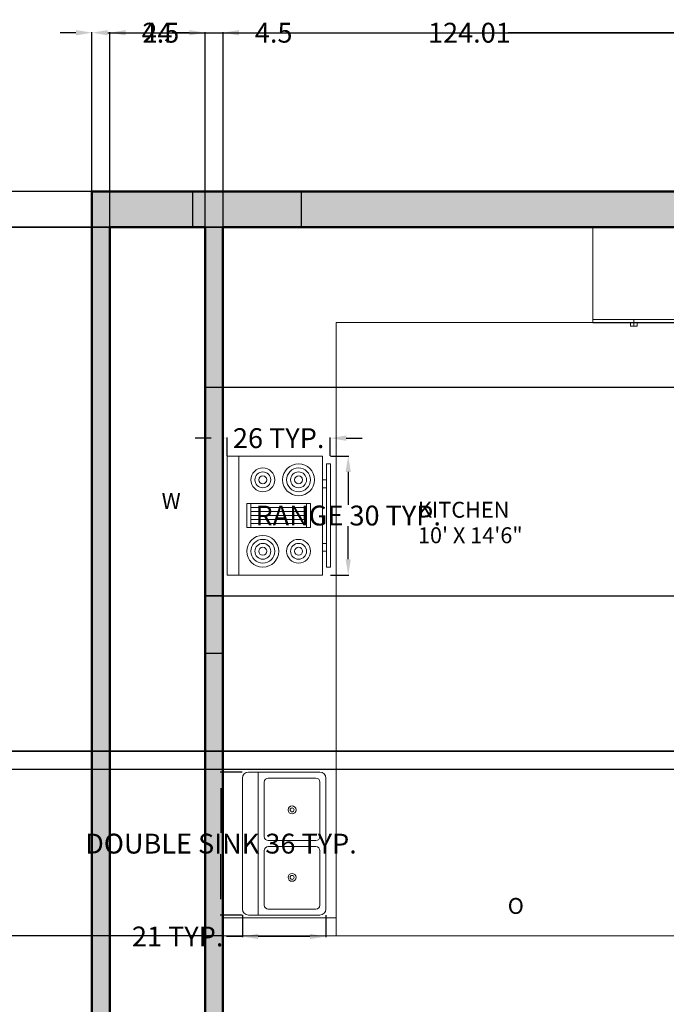
# Model space of a CAD drawing. Units: inches. Extents: x -12 to 887, y 330 to 874.
# Tile 7 of 9: x 442 to 605, y 626 to 874. Entities that reach past the tile are written whole.
import ezdxf

# ---------------------------------------------------------------- set-up
doc = ezdxf.new("R2010")
doc.units = ezdxf.units.IN
doc.header["$MEASUREMENT"] = 0
for name, color, linetype, lineweight in [('A-ANNO-DIMS', 2, 'Continuous', 18), ('A-ANNO-TEXT', 3, 'Continuous', 18), ('A-AREA-IDEN', 7, 'Continuous', 18), ('A-EQPM', 8, 'Continuous', 18), ('A-FLOR-FIXT', 8, 'Continuous', 18), ('A-GLAZ', 4, 'Continuous', 25), ('A-WALL', 7, 'Continuous', 50), ('A-WALL-PATT', 5, 'Continuous', 13)]:
    doc.layers.add(name, color=color, linetype=linetype, lineweight=lineweight)
doc.styles.get("Standard").update_dxf_attribs({"font": 'arial.ttf'})
doc.dimstyles.get("Standard").update_dxf_attribs({"dimtxt": 5, "dimasz": 4, "dimexe": 0.18, "dimexo": 0.0625, "dimgap": 0.09, "dimtad": 0, "dimtih": 1, "dimtoh": 1, "dimdec": 1, "dimzin": 0, "dimdsep": 46, "dimlunit": 4, "dimtxsty": 'Standard', "dimcen": 0.09, "dimadec": 0, "dimazin": 0, "dimtfac": 1, "dimtdec": 1, "dimtofl": 0, "dimtmove": 0, "dimatfit": 3, "dimfxl": 1, "dimtolj": 1, "dimtzin": 0, "dimarcsym": 0})

# ---------------------------------------------------------------- blocks, each defined once
blk = doc.blocks.new('Sink-double - 36 in top')
for p, q in [((-18, -4), (18, -4)), ((-0.75, -18.5), (-0.75, -6.5)), ((0.75, -6.5), (0.75, -18.5))]:
    blk.add_line(p, q)
for points in [[(-16.5, 0), (16.5, 0)], [(-18, -19.5), (-18, -1.5)], [(18, -1.5), (18, -19.5)], [(-16.5, -18.5), (-16.5, -6.5)], [(-15.5, -5.5), (-1.75, -5.5)], [(1.75, -5.5), (15.5, -5.5)], [(16.5, -6.5), (16.5, -18.5)], [(-1.75, -19.5), (-15.5, -19.5)], [(15.5, -19.5), (1.75, -19.5)], [(16.5, -21), (-16.5, -21)]]:
    blk.add_lwpolyline(points)
for centre, radius in [((-8.5, -12.5), 1), ((-8.5, -12.5), 0.5), ((8.5, -12.5), 1), ((8.5, -12.5), 0.5)]:
    blk.add_circle(centre, radius)
for centre, radius, start, end in [((-16.5, -1.5), 1.5, 90, 180), ((16.5, -1.5), 1.5, 0, 90), ((-15.5, -6.5), 1, 90, 180), ((-1.75, -6.5), 1, 0, 90), ((1.75, -6.5), 1, 90, 180), ((15.5, -6.5), 1, 0, 90), ((-16.5, -19.5), 1.5, 180, 270), ((-15.5, -18.5), 1, 180, 270), ((-1.75, -18.5), 1, 270, 0), ((1.75, -18.5), 1, 180, 270), ((15.5, -18.5), 1, 270, 0), ((16.5, -19.5), 1.5, 270, 0)]:
    blk.add_arc(centre, radius, start, end)
blk = doc.blocks.new('Range-Oven - 30 in top')
for p, q in [((0, -3), (30, -3)), ((12, -6), (18, -6)), ((13, -20), (13, -6)), ((14, -6), (14, -20)), ((15, -20), (15, -6)), ((16, -6), (16, -20)), ((17, -20), (17, -6)), ((18, -20), (12, -20)), ((6, -24), (6, -25)), ((8, -25), (8, -24)), ((22, -25), (22, -24)), ((24, -24), (24, -25))]:
    blk.add_line(p, q)
for points in [[(0, -24), (0, 0), (30, 0), (30, -24)], [(12, -21), (12, -5), (18, -5), (18, -21)], [(2, -26), (2, -25), (28, -25), (28, -26)]]:
    blk.add_lwpolyline(points, close=True)
for centre, radius in [((6, -9), 4), ((6, -9), 3), ((6, -9), 2), ((24, -9), 3), ((24, -9), 2), ((6, -9), 1), ((24, -9), 1), ((24, -18), 4), ((6, -18), 3), ((6, -18), 2), ((6, -18), 1), ((24, -18), 3), ((24, -18), 2), ((24, -18), 1)]:
    blk.add_circle(centre, radius)
blk = doc.blocks.new('Refrigerator-2 door - 36 in top')
for p, q in [((0, -26.999999), (36, -26.999999)), ((11, -27.999999), (11, -28.999999)), ((12, -26.999999), (12, -28.999999)), ((13, -28.999999), (13, -27.999999)), ((11, -28.999999), (13, -28.999999))]:
    blk.add_line(p, q)
blk.add_lwpolyline([(0, -27.999999), (0, 0), (36, 0), (36, -27.999999)], close=True)
blk = doc.blocks.new('*D24')
at = {"layer": 'A-ANNO-DIMS', "color": 0, "lineweight": -2, "transparency": 16777216}
for p, q in [((497.9, 684.39), (492.38, 684.39)), ((492.56, 680.39), (492.56, 669.07)), ((492.56, 652.39), (492.56, 663.71)), ((497.9, 648.39), (492.38, 648.39))]:
    blk.add_line(p, q, dxfattribs=at)
at = {"layer": 'A-ANNO-DIMS', "color": 0, "transparency": 16777216}
for points in [[(491.89, 680.39), (493.23, 680.39), (492.56, 684.39)], [(491.89, 652.39), (493.23, 652.39), (492.56, 648.39)]]:
    blk.add_solid(points, dxfattribs=at)
at = {"layer": 'Defpoints', "color": 0, "transparency": 16777216}
for p in [(492.56, 684.39), (497.96, 684.39), (497.96, 648.39)]:
    blk.add_point(p, dxfattribs=at)
at = {"layer": 'A-ANNO-DIMS', "color": 0, "transparency": 16777216, "insert": (492.56, 666.39), "char_height": 5, "attachment_point": 5}
blk.add_mtext('\\A1;DOUBLE SINK 36 TYP.', dxfattribs=at)
blk = doc.blocks.new('*D25')
at = {"layer": 'A-ANNO-DIMS', "color": 0, "lineweight": -2, "transparency": 16777216}
for p, q in [((497.96, 648.33), (497.96, 642.81)), ((518.96, 648.33), (518.96, 642.81)), ((497.96, 642.99), (493.96, 642.99)), ((514.96, 642.99), (501.96, 642.99))]:
    blk.add_line(p, q, dxfattribs=at)
at = {"layer": 'A-ANNO-DIMS', "color": 0, "transparency": 16777216}
for points in [[(501.96, 643.66), (501.96, 642.33), (497.96, 642.99)], [(514.96, 643.66), (514.96, 642.33), (518.96, 642.99)]]:
    blk.add_solid(points, dxfattribs=at)
at = {"layer": 'Defpoints', "color": 0, "transparency": 16777216}
for p in [(497.96, 648.39), (518.96, 648.39), (497.96, 642.99)]:
    blk.add_point(p, dxfattribs=at)
at = {"layer": 'A-ANNO-DIMS', "color": 0, "transparency": 16777216, "insert": (481.66, 642.99), "char_height": 5, "attachment_point": 5}
blk.add_mtext('\\A1;21 TYP.', dxfattribs=at)
blk = doc.blocks.new('*D26')
at = {"layer": 'A-ANNO-DIMS', "color": 0, "lineweight": -2, "transparency": 16777216}
for p, q in [((520.15, 764.03), (524.76, 764.03)), ((524.58, 760.03), (524.58, 751.71)), ((524.58, 738.03), (524.58, 746.35)), ((520.15, 734.03), (524.76, 734.03))]:
    blk.add_line(p, q, dxfattribs=at)
at = {"layer": 'A-ANNO-DIMS', "color": 0, "transparency": 16777216}
for points in [[(523.92, 760.03), (525.25, 760.03), (524.58, 764.03)], [(523.92, 738.03), (525.25, 738.03), (524.58, 734.03)]]:
    blk.add_solid(points, dxfattribs=at)
at = {"layer": 'Defpoints', "color": 0, "transparency": 16777216}
for p in [(520.08, 764.03), (524.58, 764.03), (520.08, 734.03)]:
    blk.add_point(p, dxfattribs=at)
at = {"layer": 'A-ANNO-DIMS', "color": 0, "transparency": 16777216, "insert": (524.58, 749.03), "char_height": 5, "attachment_point": 5}
blk.add_mtext('\\A1;RANGE 30 TYP.', dxfattribs=at)
blk = doc.blocks.new('*D27')
at = {"layer": 'A-ANNO-DIMS', "color": 0, "lineweight": -2, "transparency": 16777216}
for p, q in [((490.08, 768.53), (486.08, 768.53)), ((494.08, 764.09), (494.08, 768.71)), ((520.08, 764.09), (520.08, 768.71)), ((524.08, 768.53), (528.08, 768.53))]:
    blk.add_line(p, q, dxfattribs=at)
at = {"layer": 'A-ANNO-DIMS', "color": 0, "transparency": 16777216}
for points in [[(490.08, 769.2), (490.08, 767.86), (494.08, 768.53)], [(524.08, 769.2), (524.08, 767.86), (520.08, 768.53)]]:
    blk.add_solid(points, dxfattribs=at)
at = {"layer": 'Defpoints', "color": 0, "transparency": 16777216}
for p in [(494.08, 768.53), (494.08, 764.03), (520.08, 764.03)]:
    blk.add_point(p, dxfattribs=at)
at = {"layer": 'A-ANNO-DIMS', "color": 0, "transparency": 16777216, "insert": (507.08, 768.53), "char_height": 5, "attachment_point": 5}
blk.add_mtext('\\A1;26 TYP.', dxfattribs=at)
blk = doc.blocks.new('*D64')
at = {"layer": 'A-ANNO-DIMS', "color": 0, "lineweight": -2, "transparency": 16777216}
for p, q in [((383.99, 685.16), (873.75, 685.16)), ((873.57, 681.16), (873.57, 628.55)), ((873.57, 570.66), (873.57, 623.27)), ((383.99, 566.66), (873.75, 566.66))]:
    blk.add_line(p, q, dxfattribs=at)
at = {"layer": 'A-ANNO-DIMS', "color": 0, "transparency": 16777216}
for points in [[(872.9, 681.16), (874.24, 681.16), (873.57, 685.16)], [(872.9, 570.66), (874.24, 570.66), (873.57, 566.66)]]:
    blk.add_solid(points, dxfattribs=at)
at = {"layer": 'Defpoints', "color": 0, "transparency": 16777216}
for p in [(383.93, 685.16), (873.57, 685.16), (383.93, 566.66)]:
    blk.add_point(p, dxfattribs=at)
at = {"layer": 'A-ANNO-DIMS', "color": 0, "transparency": 16777216, "insert": (873.57, 625.91), "char_height": 5, "attachment_point": 5}
blk.add_mtext('\\A1;118.5', dxfattribs=at)
blk = doc.blocks.new('*D65')
at = {"layer": 'A-ANNO-DIMS', "color": 0, "lineweight": -2, "transparency": 16777216}
for p, q in [((873.57, 693.66), (873.57, 697.66)), ((873.57, 697.66), (877.57, 697.66)), ((383.99, 689.66), (873.75, 689.66)), ((383.99, 685.16), (873.75, 685.16)), ((873.57, 681.16), (873.57, 677.16))]:
    blk.add_line(p, q, dxfattribs=at)
at = {"layer": 'A-ANNO-DIMS', "color": 0, "transparency": 16777216}
for points in [[(872.9, 693.66), (874.24, 693.66), (873.57, 689.66)], [(872.9, 681.16), (874.24, 681.16), (873.57, 685.16)]]:
    blk.add_solid(points, dxfattribs=at)
at = {"layer": 'Defpoints', "color": 0, "transparency": 16777216}
for p in [(383.93, 689.66), (873.57, 689.66), (383.93, 685.16)]:
    blk.add_point(p, dxfattribs=at)
at = {"layer": 'A-ANNO-DIMS', "color": 0, "transparency": 16777216, "insert": (882.33, 697.66), "char_height": 5, "attachment_point": 5}
blk.add_mtext('\\A1;4.5', dxfattribs=at)
blk = doc.blocks.new('*D66')
at = {"layer": 'A-ANNO-DIMS', "color": 0, "lineweight": -2, "transparency": 16777216}
for p, q in [((383.99, 821.66), (873.75, 821.66)), ((873.57, 817.66), (873.57, 758.31)), ((873.57, 693.66), (873.57, 753.02)), ((383.99, 689.66), (873.75, 689.66))]:
    blk.add_line(p, q, dxfattribs=at)
at = {"layer": 'A-ANNO-DIMS', "color": 0, "transparency": 16777216}
for points in [[(872.9, 817.66), (874.24, 817.66), (873.57, 821.66)], [(872.9, 693.66), (874.24, 693.66), (873.57, 689.66)]]:
    blk.add_solid(points, dxfattribs=at)
at = {"layer": 'Defpoints', "color": 0, "transparency": 16777216}
for p in [(383.93, 821.66), (873.57, 821.66), (383.93, 689.66)]:
    blk.add_point(p, dxfattribs=at)
at = {"layer": 'A-ANNO-DIMS', "color": 0, "transparency": 16777216, "insert": (873.57, 755.66), "char_height": 5, "attachment_point": 5}
blk.add_mtext('\\A1;132', dxfattribs=at)
blk = doc.blocks.new('*D83')
at = {"layer": 'A-ANNO-DIMS', "color": 0, "lineweight": -2, "transparency": 16777216}
for p, q in [((460.07, 830.72), (460.07, 870.84)), ((464.07, 870.66), (638.28, 870.66)), ((829.57, 870.66), (655.36, 870.66)), ((833.57, 830.72), (833.57, 870.84))]:
    blk.add_line(p, q, dxfattribs=at)
at = {"layer": 'A-ANNO-DIMS', "color": 0, "transparency": 16777216}
for points in [[(464.07, 871.33), (464.07, 869.99), (460.07, 870.66)], [(829.57, 871.33), (829.57, 869.99), (833.57, 870.66)]]:
    blk.add_solid(points, dxfattribs=at)
at = {"layer": 'Defpoints', "color": 0, "transparency": 16777216}
for p in [(833.57, 870.66), (460.07, 830.66), (833.57, 830.66)]:
    blk.add_point(p, dxfattribs=at)
at = {"layer": 'A-ANNO-DIMS', "color": 0, "transparency": 16777216, "insert": (646.82, 870.66), "char_height": 5, "attachment_point": 5}
blk.add_mtext('\\A1;373.5', dxfattribs=at)
blk = doc.blocks.new('*D84')
at = {"layer": 'A-ANNO-DIMS', "color": 0, "lineweight": -2, "transparency": 16777216}
for p, q in [((456.07, 870.66), (452.07, 870.66)), ((460.07, 830.72), (460.07, 870.84)), ((464.57, 821.72), (464.57, 870.84)), ((468.57, 870.66), (472.57, 870.66))]:
    blk.add_line(p, q, dxfattribs=at)
at = {"layer": 'A-ANNO-DIMS', "color": 0, "transparency": 16777216}
for points in [[(456.07, 871.33), (456.07, 869.99), (460.07, 870.66)], [(468.57, 871.33), (468.57, 869.99), (464.57, 870.66)]]:
    blk.add_solid(points, dxfattribs=at)
at = {"layer": 'Defpoints', "color": 0, "transparency": 16777216}
for p in [(464.57, 870.66), (460.07, 830.66), (464.57, 821.66)]:
    blk.add_point(p, dxfattribs=at)
at = {"layer": 'A-ANNO-DIMS', "color": 0, "transparency": 16777216, "insert": (477.33, 870.66), "char_height": 5, "attachment_point": 5}
blk.add_mtext('\\A1;4.5', dxfattribs=at)
blk = doc.blocks.new('*D85')
at = {"layer": 'A-ANNO-DIMS', "color": 0, "lineweight": -2, "transparency": 16777216}
for p, q in [((464.57, 821.72), (464.57, 870.84)), ((468.57, 870.66), (472.86, 870.66)), ((484.57, 870.66), (480.27, 870.66)), ((488.57, 821.72), (488.57, 870.84))]:
    blk.add_line(p, q, dxfattribs=at)
at = {"layer": 'A-ANNO-DIMS', "color": 0, "transparency": 16777216}
for points in [[(468.57, 871.33), (468.57, 869.99), (464.57, 870.66)], [(484.57, 871.33), (484.57, 869.99), (488.57, 870.66)]]:
    blk.add_solid(points, dxfattribs=at)
at = {"layer": 'Defpoints', "color": 0, "transparency": 16777216}
for p in [(488.57, 870.66), (464.57, 821.66), (488.57, 821.66)]:
    blk.add_point(p, dxfattribs=at)
at = {"layer": 'A-ANNO-DIMS', "color": 0, "transparency": 16777216, "insert": (476.57, 870.66), "char_height": 5, "attachment_point": 5}
blk.add_mtext('\\A1;24', dxfattribs=at)
blk = doc.blocks.new('*D86')
at = {"layer": 'A-ANNO-DIMS', "color": 0, "lineweight": -2, "transparency": 16777216}
for p, q in [((484.57, 870.66), (480.57, 870.66)), ((488.57, 821.72), (488.57, 870.84)), ((493.07, 821.72), (493.07, 870.84)), ((497.07, 870.66), (501.07, 870.66))]:
    blk.add_line(p, q, dxfattribs=at)
at = {"layer": 'A-ANNO-DIMS', "color": 0, "transparency": 16777216}
for points in [[(484.57, 871.33), (484.57, 869.99), (488.57, 870.66)], [(497.07, 871.33), (497.07, 869.99), (493.07, 870.66)]]:
    blk.add_solid(points, dxfattribs=at)
at = {"layer": 'Defpoints', "color": 0, "transparency": 16777216}
for p in [(493.07, 870.66), (488.57, 821.66), (493.07, 821.66)]:
    blk.add_point(p, dxfattribs=at)
at = {"layer": 'A-ANNO-DIMS', "color": 0, "transparency": 16777216, "insert": (505.83, 870.66), "char_height": 5, "attachment_point": 5}
blk.add_mtext('\\A1;4.5', dxfattribs=at)
blk = doc.blocks.new('*D87')
at = {"layer": 'A-ANNO-DIMS', "color": 0, "lineweight": -2, "transparency": 16777216}
for p, q in [((493.07, 821.72), (493.07, 870.84)), ((497.07, 870.66), (545.32, 870.66)), ((613.08, 870.66), (564.83, 870.66)), ((617.08, 821.7), (617.08, 870.84))]:
    blk.add_line(p, q, dxfattribs=at)
at = {"layer": 'A-ANNO-DIMS', "color": 0, "transparency": 16777216}
for points in [[(497.07, 871.33), (497.07, 869.99), (493.07, 870.66)], [(613.08, 871.33), (613.08, 869.99), (617.08, 870.66)]]:
    blk.add_solid(points, dxfattribs=at)
at = {"layer": 'Defpoints', "color": 0, "transparency": 16777216}
for p in [(617.08, 870.66), (493.07, 821.66), (617.08, 821.64)]:
    blk.add_point(p, dxfattribs=at)
at = {"layer": 'A-ANNO-DIMS', "color": 0, "transparency": 16777216, "insert": (555.08, 870.66), "char_height": 5, "attachment_point": 5}
blk.add_mtext('\\A1;124.01', dxfattribs=at)
blk = doc.blocks.new('*D98')
at = {"layer": 'A-ANNO-DIMS', "color": 0, "lineweight": -2, "transparency": 16777216}
for p, q in [((460.13, 830.66), (873.75, 830.66)), ((873.57, 826.66), (873.57, 604.54)), ((873.57, 377.16), (873.57, 599.28)), ((460.13, 373.16), (873.75, 373.16))]:
    blk.add_line(p, q, dxfattribs=at)
at = {"layer": 'A-ANNO-DIMS', "color": 0, "transparency": 16777216}
for points in [[(872.9, 826.66), (874.24, 826.66), (873.57, 830.66)], [(872.9, 377.16), (874.24, 377.16), (873.57, 373.16)]]:
    blk.add_solid(points, dxfattribs=at)
at = {"layer": 'Defpoints', "color": 0, "transparency": 16777216}
for p in [(460.07, 830.66), (873.57, 830.66), (460.07, 373.16)]:
    blk.add_point(p, dxfattribs=at)
at = {"layer": 'A-ANNO-DIMS', "color": 0, "transparency": 16777216, "insert": (873.57, 601.91), "char_height": 5, "attachment_point": 5}
blk.add_mtext('\\A1;457.5', dxfattribs=at)
blk = doc.blocks.new('*D101')
at = {"layer": 'A-ANNO-DIMS', "color": 0, "lineweight": -2, "transparency": 16777216}
for p, q in [((493.01, 643.16), (1.75, 643.16)), ((1.93, 639.16), (1.93, 551.3)), ((1.93, 458.16), (1.93, 546.02)), ((493.01, 454.16), (1.75, 454.16))]:
    blk.add_line(p, q, dxfattribs=at)
at = {"layer": 'A-ANNO-DIMS', "color": 0, "transparency": 16777216}
for points in [[(1.26, 639.16), (2.59, 639.16), (1.93, 643.16)], [(1.26, 458.16), (2.59, 458.16), (1.93, 454.16)]]:
    blk.add_solid(points, dxfattribs=at)
at = {"layer": 'Defpoints', "color": 0, "transparency": 16777216}
for p in [(1.93, 643.16), (493.07, 643.16), (493.07, 454.16)]:
    blk.add_point(p, dxfattribs=at)
at = {"layer": 'A-ANNO-DIMS', "color": 0, "transparency": 16777216, "insert": (1.93, 548.66), "char_height": 5, "attachment_point": 5}
blk.add_mtext('\\A1;189', dxfattribs=at)
blk = doc.blocks.new('*D102')
at = {"layer": 'A-ANNO-DIMS', "color": 0, "lineweight": -2, "transparency": 16777216}
for p, q in [((493.01, 821.66), (1.75, 821.66)), ((1.93, 817.66), (1.93, 735.05)), ((1.93, 647.16), (1.93, 729.77)), ((493.01, 643.16), (1.75, 643.16))]:
    blk.add_line(p, q, dxfattribs=at)
at = {"layer": 'A-ANNO-DIMS', "color": 0, "transparency": 16777216}
for points in [[(1.26, 817.66), (2.59, 817.66), (1.93, 821.66)], [(1.26, 647.16), (2.59, 647.16), (1.93, 643.16)]]:
    blk.add_solid(points, dxfattribs=at)
at = {"layer": 'Defpoints', "color": 0, "transparency": 16777216}
for p in [(1.93, 821.66), (493.07, 821.66), (493.07, 643.16)]:
    blk.add_point(p, dxfattribs=at)
at = {"layer": 'A-ANNO-DIMS', "color": 0, "transparency": 16777216, "insert": (1.93, 732.41), "char_height": 5, "attachment_point": 5}
blk.add_mtext('\\A1;178.5', dxfattribs=at)
blk = doc.blocks.new('*D103')
at = {"layer": 'A-ANNO-DIMS', "color": 0, "lineweight": -2, "transparency": 16777216}
for p, q in [((1.93, 830.66), (1.93, 834.66)), ((1.93, 834.66), (5.93, 834.66)), ((460.01, 830.66), (1.75, 830.66)), ((1.93, 825.66), (1.93, 826.66)), ((493.01, 821.66), (1.75, 821.66))]:
    blk.add_line(p, q, dxfattribs=at)
at = {"layer": 'A-ANNO-DIMS', "color": 0, "transparency": 16777216}
for points in [[(1.26, 826.66), (2.59, 826.66), (1.93, 830.66)], [(1.26, 825.66), (2.59, 825.66), (1.93, 821.66)]]:
    blk.add_solid(points, dxfattribs=at)
at = {"layer": 'Defpoints', "color": 0, "transparency": 16777216}
for p in [(1.93, 830.66), (460.07, 830.66), (493.07, 821.66)]:
    blk.add_point(p, dxfattribs=at)
at = {"layer": 'A-ANNO-DIMS', "color": 0, "transparency": 16777216, "insert": (7.66, 834.66), "char_height": 5, "attachment_point": 5}
blk.add_mtext('\\A1;9', dxfattribs=at)
blk = doc.blocks.new('*D112')
at = {"layer": 'A-ANNO-DIMS', "color": 0, "lineweight": -2, "transparency": 16777216}
for p, q in [((676.01, 821.66), (1.75, 821.66)), ((1.93, 817.66), (1.93, 758.31)), ((1.93, 693.66), (1.93, 753.02)), ((676.01, 689.66), (1.75, 689.66))]:
    blk.add_line(p, q, dxfattribs=at)
at = {"layer": 'A-ANNO-DIMS', "color": 0, "transparency": 16777216}
for points in [[(1.26, 817.66), (2.59, 817.66), (1.93, 821.66)], [(1.26, 693.66), (2.59, 693.66), (1.93, 689.66)]]:
    blk.add_solid(points, dxfattribs=at)
at = {"layer": 'Defpoints', "color": 0, "transparency": 16777216}
for p in [(1.93, 821.66), (676.07, 821.66), (676.07, 689.66)]:
    blk.add_point(p, dxfattribs=at)
at = {"layer": 'A-ANNO-DIMS', "color": 0, "transparency": 16777216, "insert": (1.93, 755.66), "char_height": 5, "attachment_point": 5}
blk.add_mtext('\\A1;132', dxfattribs=at)
blk = doc.blocks.new('*D128')
at = {"layer": 'A-ANNO-DIMS', "color": 0, "lineweight": -2, "transparency": 16777216}
for p, q in [((488.63, 781.36), (873.75, 781.36)), ((873.57, 777.36), (873.57, 757.74)), ((873.57, 732.83), (873.57, 752.45)), ((488.63, 728.83), (873.75, 728.83))]:
    blk.add_line(p, q, dxfattribs=at)
at = {"layer": 'A-ANNO-DIMS', "color": 0, "transparency": 16777216}
for points in [[(872.9, 777.36), (874.24, 777.36), (873.57, 781.36)], [(872.9, 732.83), (874.24, 732.83), (873.57, 728.83)]]:
    blk.add_solid(points, dxfattribs=at)
at = {"layer": 'Defpoints', "color": 0, "transparency": 16777216}
for p in [(488.57, 781.36), (488.57, 728.83), (873.57, 728.83)]:
    blk.add_point(p, dxfattribs=at)
at = {"layer": 'A-ANNO-DIMS', "color": 0, "transparency": 16777216, "insert": (873.57, 755.1), "char_height": 5, "attachment_point": 5}
blk.add_mtext('\\A1;52.54', dxfattribs=at)

msp = doc.modelspace()

# ---------------------------------------------------------------- hatches: boundary and pattern name
at = {"layer": 'A-WALL-PATT'}
h = msp.add_hatch(color=256, dxfattribs=at)
h.dxf.hatch_style = 1
h.paths.add_polyline_path([(94.575, 830.6611), (67.3199, 830.6611), (67.3199, 821.6611), (70.4263, 821.6611), (79.4263, 821.6611), (94.575, 821.6611)])
h.paths.add_polyline_path([(288.8031, 830.6611), (257.9263, 830.6611), (253.4263, 830.6611), (253.4263, 821.6611), (288.8031, 821.6611)])
h.paths.add_polyline_path([(74.9263, 696.9265), (70.4263, 696.9265), (70.4263, 678.4656), (74.9263, 678.4656)])
h.paths.add_polyline_path([(74.9263, 584.8756), (70.4263, 584.8756), (70.4263, 562.1611), (74.9263, 562.1611)])
h.paths.add_polyline_path([(135.5357, 566.6611), (122.6994, 566.6611), (122.6994, 562.1611), (135.5357, 562.1611)])
h.paths.add_polyline_path([(257.9263, 579.1607), (253.4263, 579.1607), (253.4263, 562.1611), (257.9263, 562.1611)])
h.paths.add_polyline_path([(272.0195, 454.1611), (254.2006, 454.1611), (254.2006, 450.1611), (272.0195, 450.1611)])
h.paths.add_polyline_path([(392.9263, 454.1611), (374.959, 454.1611), (374.959, 450.1611), (383.9263, 450.1611), (392.9263, 450.1611)])
h.paths.add_polyline_path([(493.0683, 466.4171), (488.5683, 466.4171), (488.5683, 450.1611), (493.0683, 450.1611)])
h.paths.add_polyline_path([(568.6302, 454.1611), (555.938, 454.1611), (555.938, 450.1611), (568.6302, 450.1611)])
h.paths.add_polyline_path([(493.0683, 594.9471), (488.5683, 594.9471), (488.5683, 569.5862), (493.0683, 569.5862)])
h.paths.add_polyline_path([(690.1615, 454.1611), (672.3426, 454.1611), (672.3426, 450.1611), (690.1615, 450.1611)])
h.paths.add_polyline_path([(811.0683, 454.1611), (793.101, 454.1611), (793.101, 450.1611), (802.0683, 450.1611), (811.0683, 450.1611)])
h.paths.add_polyline_path([(811.0683, 578.3606), (802.0683, 578.3606), (802.0683, 566.6611), (802.0683, 553.5254), (811.0683, 553.5254)])
h.paths.add_polyline_path([(811.0683, 701.6611), (802.0683, 701.6611), (802.0683, 689.9616), (802.0683, 676.8259), (811.0683, 676.8259)])
h.paths.add_polyline_path([(811.0683, 830.6611), (782.165, 830.6611), (782.165, 821.6611), (802.0683, 821.6611), (811.0683, 821.6611)])
h.paths.add_polyline_path([(706.9451, 830.6611), (671.5683, 830.6611), (671.5683, 821.6611), (706.9451, 821.6611)])
h.paths.add_polyline_path([(512.717, 830.6611), (485.4619, 830.6611), (485.4619, 821.6611), (488.5683, 821.6611), (512.717, 821.6611)])
h.paths.add_polyline_path([(392.9263, 697.8668), (383.9263, 697.8668), (383.9263, 689.6611), (383.9263, 676.5034), (392.9263, 676.5034)])
h.paths.add_polyline_path([(392.9263, 830.6611), (364.023, 830.6611), (364.023, 821.7357), (392.9263, 821.7357)])
h.paths.add_polyline_path([(392.9263, 619.0434), (383.9263, 619.0434), (383.9263, 588.7499), (392.9263, 588.7499)])
h.paths.add_polyline_path([(392.9263, 578.3606), (383.9263, 578.3606), (383.9263, 566.6611), (383.9263, 553.5254), (392.9263, 553.5254)])
h.paths.add_polyline_path([(257.9263, 699.8547), (253.4263, 699.8547), (253.4263, 697.1611), (253.4263, 677.338), (257.9263, 677.338)])
h.paths.add_polyline_path([(493.0683, 714.3785), (488.5683, 714.3785), (488.5683, 689.6611), (493.0683, 689.6611)])
h.paths.add_polyline_path([(74.9263, 491.4191), (70.4263, 491.4191), (70.4263, 480.7097), (74.9263, 480.7097)])
h = msp.add_hatch(color=256, dxfattribs=at)
h.dxf.hatch_style = 1
h.paths.add_polyline_path([(671.5683, 830.6611), (512.717, 830.6611), (512.717, 821.6611), (617.0825, 821.6611), (617.0825, 797.5825), (617.0787, 783.3094), (621.5683, 783.3094), (621.5683, 821.6611), (671.5683, 821.6611)], flags=17)
h.paths.add_polyline_path([(833.5683, 830.6611), (811.0683, 830.6611), (811.0683, 821.6611), (829.0683, 821.6611), (829.0683, 701.6611), (829.0683, 382.1611), (811.0683, 382.1611), (811.0683, 450.1611), (802.0683, 450.1611), (802.0683, 382.1611), (671.5683, 382.1611), (464.5683, 382.1611), (464.5683, 821.6611), (460.0683, 821.6611), (460.0683, 373.1611), (671.5683, 373.1611), (833.5683, 373.1611)])
h.paths.add_polyline_path([(493.0683, 728.8273), (488.5683, 728.8273), (488.5683, 714.3785), (493.0683, 714.3785)], flags=17)
h.paths.add_polyline_path([(493.0683, 821.6611), (488.5683, 821.6611), (488.5683, 781.3634), (493.0683, 781.3634)], flags=17)
h = msp.add_hatch(color=256, dxfattribs=at)
h.dxf.hatch_style = 1
h.paths.add_polyline_path([(485.4619, 830.6611), (460.0683, 830.6611), (460.0683, 373.1611), (833.5683, 373.1611), (833.5683, 830.6611), (811.0683, 830.6611), (811.0683, 821.6611), (829.0683, 821.6611), (829.0683, 701.6611), (829.0683, 382.1611), (811.0683, 382.1611), (811.0683, 450.1611), (802.0683, 450.1611), (802.0683, 382.1611), (671.5683, 382.1611), (464.5683, 382.1611), (464.5683, 821.6611), (485.4619, 821.6611)])
h = msp.add_hatch(color=256, dxfattribs=at)
h.dxf.hatch_style = 1
h.paths.add_polyline_path([(671.5683, 749.6611), (621.5683, 749.6611), (621.5683, 759.3094), (620.6653, 759.3094), (617.0683, 759.3094), (617.0683, 745.1611), (671.5683, 745.1611)])
h.paths.add_polyline_path([(676.0683, 821.6611), (671.5683, 821.6611), (671.5683, 736.2424), (676.0683, 736.2424)])
h.paths.add_polyline_path([(782.165, 830.6611), (706.9451, 830.6611), (706.9451, 821.6611), (782.165, 821.6611)])
h.paths.add_polyline_path([(811.0683, 553.5254), (802.0683, 553.5254), (802.0683, 507.4529), (802.0683, 454.1611), (811.0683, 454.1611)])
h.paths.add_polyline_path([(793.101, 454.1611), (690.1615, 454.1611), (690.1615, 450.1611), (793.101, 450.1611)])
h.paths.add_polyline_path([(672.3426, 454.1611), (656.7304, 454.1611), (656.7304, 450.1611), (672.3426, 450.1611)])
h.paths.add_polyline_path([(582.6585, 454.1611), (568.6302, 454.1611), (568.6302, 450.1611), (582.6585, 450.1611)])
h.paths.add_polyline_path([(555.938, 454.1611), (554.2565, 454.1611), (554.2565, 452.8628), (554.2565, 450.1611), (555.938, 450.1611)])
h.paths.add_polyline_path([(518.2335, 452.8628), (518.2335, 454.1611), (493.0683, 454.1611), (493.0683, 450.1611), (518.2335, 450.1611)])
h.paths.add_polyline_path([(493.0683, 450.1611), (488.5683, 450.1611), (488.5683, 382.1611), (493.0683, 382.1611)])
h.paths.add_polyline_path([(493.0683, 492.3446), (488.5683, 492.3446), (488.5683, 466.4171), (493.0683, 466.4171)])
h.paths.add_polyline_path([(493.0683, 569.5862), (488.5683, 569.5862), (488.5683, 557.2595), (493.0683, 557.2595)])
h.paths.add_polyline_path([(493.0683, 689.6611), (488.5683, 689.6611), (488.5683, 594.9471), (493.0683, 594.9471)])
h.paths.add_polyline_path([(676.0683, 700.2227), (671.5683, 700.2227), (671.5683, 669.5589), (676.0683, 669.5589)])
h.paths.add_polyline_path([(739.0683, 689.6611), (676.0683, 689.6611), (676.0683, 685.1611), (739.0683, 685.1611)])
h.paths.add_polyline_path([(802.0683, 689.6611), (763.0683, 689.6611), (763.0683, 686.0698), (763.0683, 685.1611), (802.0683, 685.1611)])
h.paths.add_polyline_path([(811.0683, 821.6611), (802.0683, 821.6611), (802.0683, 756.0738), (811.0683, 756.0738)])
h.paths.add_polyline_path([(811.0683, 707.8935), (802.0683, 707.8935), (802.0683, 701.6611), (811.0683, 701.6611)])
h.paths.add_polyline_path([(811.0683, 676.8259), (802.0683, 676.8259), (802.0683, 628.1611), (730.0683, 628.1611), (730.0683, 623.6611), (802.0683, 623.6611), (802.0683, 578.3606), (811.0683, 578.3606)])
h.paths.add_polyline_path([(730.0683, 685.1611), (726.0683, 685.1611), (726.0683, 628.1611), (730.0683, 628.1611)])
h.paths.add_polyline_path([(724.0683, 685.1611), (720.0683, 685.1611), (720.0683, 628.1611), (724.0683, 628.1611)])
h.paths.add_polyline_path([(726.0683, 628.1611), (676.0683, 628.1611), (676.0683, 633.7662), (674.2492, 633.7662), (671.5683, 633.7662), (671.5683, 623.6611), (726.0683, 623.6611)])
h.paths.add_polyline_path([(730.0683, 628.1611), (726.0683, 628.1611), (726.0683, 623.6611), (730.0683, 623.6611)])
h.paths.add_polyline_path([(730.0683, 623.6611), (726.0683, 623.6611), (726.0683, 595.3822), (729.6731, 595.3822, -0.00411226), (730.0683, 595.379)])
h.paths.add_polyline_path([(802.0683, 564.6611), (730.0683, 564.6611), (730.0683, 571.3507), (729.6731, 571.3507), (726.0683, 571.3507), (726.0683, 564.6611), (718.522, 564.6611), (718.522, 560.1611), (802.0683, 560.1611)])
h.paths.add_polyline_path([(676.0683, 580.4772), (671.5683, 580.4772), (671.5683, 560.1611), (676.0683, 560.1611)])
h.paths.add_polyline_path([(682.5176, 564.6611), (676.0683, 564.6611), (676.0683, 560.1611), (682.5176, 560.1611)])
h.paths.add_polyline_path([(676.0683, 560.1611), (671.5683, 560.1611), (671.5683, 454.1611), (672.3426, 454.1611), (676.0683, 454.1611)])
h = msp.add_hatch(color=256, dxfattribs=at)
h.dxf.hatch_style = 1
h.paths.add_polyline_path([(74.9263, 749.8953), (70.4263, 749.8953), (70.4263, 709.2627), (74.9263, 709.2627)])
h.paths.add_polyline_path([(74.9263, 671.2153), (70.4263, 671.2153), (70.4263, 599.271), (74.9263, 599.271)])
h.paths.add_polyline_path([(229.0035, 566.6611), (142.5107, 566.6611), (142.5107, 562.1611), (229.0035, 562.1611)])
h.paths.add_polyline_path([(392.9263, 742.7561), (383.9263, 742.7561), (383.9263, 706.6608), (392.9263, 706.6608)])
h.paths.add_polyline_path([(656.7304, 454.1611), (582.6585, 454.1611), (582.6585, 450.1611), (656.7304, 450.1611)])
h.paths.add_polyline_path([(493.0683, 557.2595), (488.5683, 557.2595), (488.5683, 492.3446), (493.0683, 492.3446)])
h.paths.add_polyline_path([(493.0683, 781.3634), (488.5683, 781.3634), (488.5683, 728.8273), (493.0683, 728.8273)])
h.paths.add_polyline_path([(811.0683, 756.0738), (802.0683, 756.0738), (802.0683, 707.8935), (811.0683, 707.8935)])

# ---------------------------------------------------------------- linework, layer by layer
at = {"layer": 'A-FLOR-FIXT'}
for p, q in [((521.5683, 797.6611), (617.0683, 797.6611)), ((521.5683, 797.6611), (521.5683, 643.1611)), ((493.0683, 647.6611), (521.5683, 647.6611)), ((493.0683, 643.1611), (617.0683, 643.1611))]:
    msp.add_line(p, q, dxfattribs=at)
at = {"layer": 'A-GLAZ'}
msp.add_lwpolyline([(488.5683, 821.6611), (485.4619, 821.6611), (485.4619, 830.6611), (512.717, 830.6611), (512.717, 821.6611), (485.4619, 821.6611)], dxfattribs=at)
for points in [[(493.0683, 728.8273), (488.5683, 728.8273), (488.5683, 781.3634), (493.0683, 781.3634)], [(493.0683, 689.6611), (488.5683, 689.6611), (488.5683, 714.3785), (493.0683, 714.3785)]]:
    msp.add_lwpolyline(points, close=True, dxfattribs=at)
at = {"layer": 'A-WALL'}
for p, q in [((460.0683, 830.6611), (460.0683, 373.1611)), ((460.0683, 830.6611), (671.5683, 830.6611)), ((460.0683, 821.659), (460.0683, 373.1611)), ((464.5683, 821.6611), (464.5683, 382.1611)), ((464.5683, 821.6611), (488.5683, 821.6611)), ((464.5683, 382.1611), (464.5683, 821.6611)), ((488.5683, 821.6611), (488.5683, 382.1611)), ((493.0683, 821.6611), (493.0683, 689.6611)), ((493.0683, 821.6611), (493.0683, 382.1611)), ((493.0683, 821.6611), (497.5683, 821.6611)), ((497.5683, 821.6611), (617.0683, 821.6611))]:
    msp.add_line(p, q, dxfattribs=at)

# ---------------------------------------------------------------- block references
at = {"layer": 'A-EQPM', "xscale": 0.8591090410497297, "yscale": 0.8591090410497297, "zscale": 0.8591090410497297}
msp.add_blockref('Refrigerator-2 door - 36 in top', (586.1546, 821.6375), dxfattribs=at)
at = {"layer": 'A-EQPM', "rotation": 90}
msp.add_blockref('Range-Oven - 30 in top', (494.0849, 734.0307), dxfattribs=at)
at = {"layer": 'A-FLOR-FIXT', "rotation": 90}
msp.add_blockref('Sink-double - 36 in top', (497.9605, 666.392), dxfattribs=at)

# ---------------------------------------------------------------- texts
at = {"layer": 'A-ANNO-TEXT'}
for s, p in [('W', (477.6278, 750.724)), ('O ', (564.7341, 648.6922))]:
    msp.add_text(s, height=4, dxfattribs=at).set_placement(p)
at = {"layer": 'A-AREA-IDEN'}
for s, p in [('KITCHEN', (542.1354, 748.4934)), ('10\' X 14\'6"', (542.1354, 742.0677))]:
    msp.add_text(s, height=4, dxfattribs=at).set_placement(p)

# ---------------------------------------------------------------- dimensions: what is measured, and where the dimension line sits
at = {"layer": 'A-ANNO-DIMS'}
for base, p1, p2, override, picture, middle in [((464.5683, 870.6611), (460.0683, 830.6611), (464.5683, 821.6611), {"dimdec": 1, "dimlfac": 1, "dimrnd": 0, "dimzin": 0, "dimdsep": 46, "dimlunit": 2}, '*D84', (477.3292, 870.6611)), ((833.5683, 870.6611), (460.0683, 830.6611), (833.5683, 830.6611), {"dimdec": 1, "dimlfac": 1, "dimrnd": 0, "dimzin": 0, "dimdsep": 46, "dimlunit": 2}, '*D83', (646.8183, 870.6611)), ((488.5683, 870.6611), (464.5683, 821.6611), (488.5683, 821.6611), {"dimdec": 0, "dimlfac": 1, "dimrnd": 0, "dimzin": 0, "dimdsep": 46, "dimlunit": 2}, '*D85', (476.5683, 870.6611)), ((493.0683, 870.6611), (488.5683, 821.6611), (493.0683, 821.6611), {"dimdec": 1, "dimlfac": 1, "dimrnd": 0, "dimzin": 0, "dimdsep": 46, "dimlunit": 2}, '*D86', (505.8292, 870.6611)), ((617.0825, 870.6611), (493.0683, 821.6611), (617.0825, 821.6375), {"dimdec": 2, "dimlfac": 1, "dimrnd": 0, "dimzin": 0, "dimdsep": 46, "dimlunit": 2}, '*D87', (555.0754, 870.6611))]:
    dim = msp.add_linear_dim(base=base, p1=p1, p2=p2, dimstyle='Standard', override=override, dxfattribs=at)
    dim.commit()
    dim.dimension.update_dxf_attribs({"geometry": picture, "text_midpoint": middle})
for base, p1, p2, override, picture, middle in [((1.9263, 830.6611), (493.0683, 821.6611), (460.0683, 830.6611), {"dimdec": 0, "dimlfac": 1, "dimrnd": 0, "dimzin": 0, "dimdsep": 46, "dimlunit": 2}, '*D103', (7.6603, 834.6611)), ((873.5683, 830.6611), (460.0683, 373.1611), (460.0683, 830.6611), {"dimdec": 1, "dimlfac": 1, "dimrnd": 0, "dimzin": 0, "dimdsep": 46, "dimlunit": 2}, '*D98', (873.5683, 601.9111)), ((1.9263, 821.6611), (493.0683, 643.1611), (493.0683, 821.6611), {"dimdec": 1, "dimlfac": 1, "dimrnd": 0, "dimzin": 0, "dimdsep": 46, "dimlunit": 2}, '*D102', (1.9263, 732.4111)), ((1.9263, 821.6611), (676.0683, 689.6611), (676.0683, 821.6611), {"dimdec": 0, "dimlfac": 1, "dimrnd": 0, "dimzin": 0, "dimdsep": 46, "dimlunit": 2}, '*D112', (1.9263, 755.6611)), ((873.5683, 821.6611), (383.9263, 689.6611), (383.9263, 821.6611), {"dimdec": 0, "dimlfac": 1, "dimrnd": 0, "dimzin": 0, "dimdsep": 46, "dimlunit": 2}, '*D66', (873.5683, 755.6611)), ((873.5683, 728.8273), (488.5683, 781.3634), (488.5683, 728.8273), {"dimdec": 2, "dimlfac": 1, "dimrnd": 0, "dimzin": 0, "dimdsep": 46, "dimlunit": 2}, '*D128', (873.5683, 755.0953)), ((873.5683, 689.6611), (383.9263, 685.1611), (383.9263, 689.6611), {"dimdec": 1, "dimlfac": 1, "dimrnd": 0, "dimzin": 0, "dimdsep": 46, "dimlunit": 2}, '*D65', (882.3292, 697.6611)), ((873.5683, 685.1611), (383.9263, 566.6611), (383.9263, 685.1611), {"dimdec": 1, "dimlfac": 1, "dimrnd": 0, "dimzin": 0, "dimdsep": 46, "dimlunit": 2}, '*D64', (873.5683, 625.9111)), ((1.9263, 643.1611), (493.0683, 454.1611), (493.0683, 643.1611), {"dimdec": 0, "dimlfac": 1, "dimrnd": 0, "dimzin": 0, "dimdsep": 46, "dimlunit": 2}, '*D101', (1.9263, 548.6611))]:
    dim = msp.add_linear_dim(base=base, p1=p1, p2=p2, angle=90, dimstyle='Standard', override=override, dxfattribs=at)
    dim.commit()
    dim.dimension.update_dxf_attribs({"geometry": picture, "text_midpoint": middle})
for base, p1, p2, angle, text, picture, middle in [((494.0849, 768.5307), (520.0849, 764.0307), (494.0849, 764.0307), 180, '<> TYP.', '*D27', (507.0849, 768.5307)), ((524.5849, 764.0307), (520.0849, 734.0307), (520.0849, 764.0307), 90, 'RANGE <> TYP.', '*D26', (524.5849, 749.0307)), ((492.5605, 684.392), (497.9605, 648.392), (497.9605, 684.392), 90, 'DOUBLE SINK <> TYP.', '*D24', (492.5605, 666.392)), ((497.9605, 642.992), (518.9605, 648.392), (497.9605, 648.392), 180, '<> TYP.', '*D25', (481.6587, 642.992))]:
    dim = msp.add_linear_dim(base=base, p1=p1, p2=p2, angle=angle, text=text, dimstyle='Standard', override={"dimdec": 0, "dimrnd": 0, "dimzin": 0, "dimlunit": 2}, dxfattribs=at)
    dim.commit()
    dim.dimension.update_dxf_attribs({"geometry": picture, "text_midpoint": middle})

doc.saveas('drawing.dxf')
